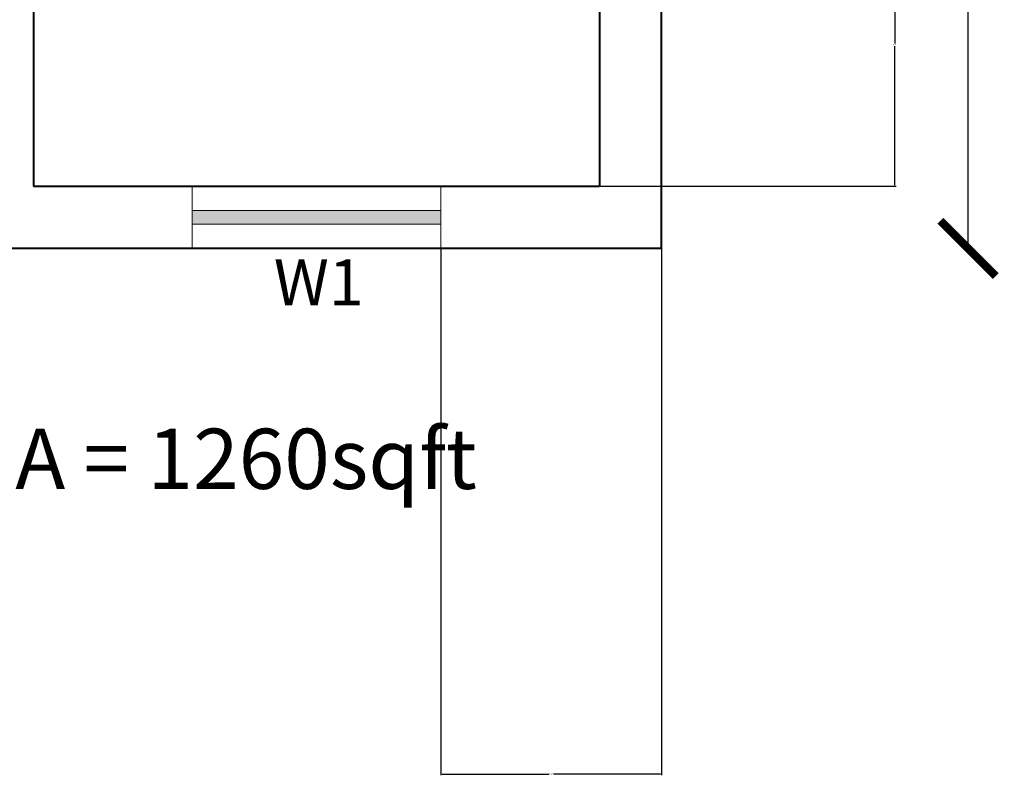
# Model space of a CAD drawing. Units: inches. Extents: x 182 to 1022, y -617 to 111.
# Tile 24 of 33: x 879 to 1022, y -617 to -507. Entities that reach past the tile are written whole.
import ezdxf

# ---------------------------------------------------------------- set-up
doc = ezdxf.new("R2010")
doc.units = ezdxf.units.IN
doc.header["$MEASUREMENT"] = 0
for name, color, linetype, lineweight in [('A-ANNO-DIMS', 2, 'Continuous', 18), ('A-ANNO-IDEN', 1, 'Continuous', 18), ('A-ANNO-TEXT', 8, 'Continuous', 20), ('A-GLAZ-PATT', 5, 'Continuous', 13), ('wall', 1, 'Continuous', 40), ('wind', 5, 'Continuous', 20)]:
    doc.layers.add(name, color=color, linetype=linetype, lineweight=lineweight)
doc.styles.get("Standard").update_dxf_attribs({"font": 'arial.ttf'})
doc.dimstyles.get("Standard").update_dxf_attribs({"dimtxt": 0.18, "dimasz": 0.18, "dimexe": 0.18, "dimexo": 0.0625, "dimgap": 0.09, "dimtad": 0, "dimtih": 1, "dimtoh": 1, "dimdec": 1, "dimzin": 0, "dimdsep": 46, "dimlunit": 4, "dimtxsty": 'Standard', "dimcen": 0.09, "dimadec": 0, "dimazin": 0, "dimtfac": 1, "dimtdec": 1, "dimtofl": 0, "dimtmove": 0, "dimatfit": 3, "dimfxl": 1, "dimtolj": 1, "dimtzin": 0, "dimarcsym": 0})

# ---------------------------------------------------------------- blocks, each defined once
blk = doc.blocks.new('_ArchTick')
at = {"color": 0, "linetype": 'ByBlock', "const_width": 0.15}
blk.add_lwpolyline([(-0.5, -0.5), (0.5, 0.5)], dxfattribs=at)
blk = doc.blocks.new('*D8')
at = {"layer": 'A-ANNO-DIMS', "color": 0, "lineweight": -2, "transparency": 16777216}
for p, q in [((1016.69, -0.37), (1016.69, -260.42)), ((1016.69, -540.37), (1016.69, -280.32))]:
    blk.add_line(p, q, dxfattribs=at)
at = {"layer": 'Defpoints', "color": 0, "transparency": 16777216}
for p in [(972.3, -0.37), (972.3, -540.37), (1016.69, -540.37)]:
    blk.add_point(p, dxfattribs=at)
at = {"layer": 'A-ANNO-DIMS', "color": 0, "lineweight": -2, "transparency": 16777216, "xscale": 8, "yscale": 8, "zscale": 8}
for p, rotation in [((1016.69, -0.37), 90), ((1016.69, -540.37), 270)]:
    blk.add_blockref('_ArchTick', p, dxfattribs=dict(at, rotation=rotation))
at = {"layer": 'A-ANNO-DIMS', "color": 0, "transparency": 16777216, "insert": (1016.69, -270.37), "char_height": 8, "attachment_point": 5, "rotation": 90}
blk.add_mtext("\\A1;45'", dxfattribs=at)
blk = doc.blocks.new('*D40')
at = {"layer": 'A-ANNO-DIMS', "color": 0, "lineweight": -2, "transparency": 16777216}
for p, q in [((940.3, -540.44), (940.3, -616.67)), ((972.3, -540.44), (972.3, -616.67)), ((940.48, -616.49), (955.97, -616.49)), ((972.12, -616.49), (956.64, -616.49))]:
    blk.add_line(p, q, dxfattribs=at)
at = {"layer": 'A-ANNO-DIMS', "color": 0, "transparency": 16777216}
for points in [[(940.48, -616.46), (940.48, -616.52), (940.3, -616.49)], [(972.12, -616.46), (972.12, -616.52), (972.3, -616.49)]]:
    blk.add_solid(points, dxfattribs=at)
at = {"layer": 'Defpoints', "color": 0, "transparency": 16777216}
for p in [(940.3, -540.37), (972.3, -540.37), (972.3, -616.49)]:
    blk.add_point(p, dxfattribs=at)
at = {"layer": 'A-ANNO-DIMS', "color": 0, "transparency": 16777216, "insert": (956.3, -616.49), "char_height": 0.18, "attachment_point": 5}
blk.add_mtext('\\A1;2\'-8"', dxfattribs=at)
blk = doc.blocks.new('*D45')
at = {"layer": 'A-ANNO-DIMS', "color": 0, "lineweight": -2, "transparency": 16777216}
for p, q in [((963.37, -490.37), (1006.28, -490.37)), ((1006.1, -490.55), (1006.1, -510.69)), ((1006.1, -531.19), (1006.1, -511.06)), ((963.37, -531.37), (1006.28, -531.37))]:
    blk.add_line(p, q, dxfattribs=at)
at = {"layer": 'A-ANNO-DIMS', "color": 0, "transparency": 16777216}
for points in [[(1006.07, -490.55), (1006.13, -490.55), (1006.1, -490.37)], [(1006.07, -531.19), (1006.13, -531.19), (1006.1, -531.37)]]:
    blk.add_solid(points, dxfattribs=at)
at = {"layer": 'Defpoints', "color": 0, "transparency": 16777216}
for p in [(963.3, -490.37), (963.3, -531.37), (1006.1, -531.37)]:
    blk.add_point(p, dxfattribs=at)
at = {"layer": 'A-ANNO-DIMS', "color": 0, "transparency": 16777216, "insert": (1006.1, -510.87), "char_height": 0.18, "attachment_point": 5}
blk.add_mtext('\\A1;3\'-5"', dxfattribs=at)

msp = doc.modelspace()

# ---------------------------------------------------------------- hatches: boundary and pattern name
at = {"layer": 'A-GLAZ-PATT'}
h = msp.add_hatch(color=256, dxfattribs=at)
h.dxf.hatch_style = 1
h.paths.add_polyline_path([(692.35, -3.87), (662.35, -3.87), (662.35, -5.87), (692.35, -5.87)])
h.paths.add_polyline_path([(783.03, -3.87), (747.03, -3.87), (747.03, -5.87), (783.03, -5.87)])
h.paths.add_polyline_path([(641.8, -252.37), (639.8, -252.37), (639.8, -288.37), (641.8, -288.37)])
h.paths.add_polyline_path([(968.8, -258.37), (966.8, -258.37), (966.8, -282.37), (968.8, -282.37)])
h.paths.add_polyline_path([(968.8, -132.92), (966.8, -132.92), (966.8, -168.92), (968.8, -168.92)])
h.paths.add_polyline_path([(940.3, -534.87), (904.3, -534.87), (904.3, -536.87), (940.3, -536.87)])

# ---------------------------------------------------------------- linework, layer by layer
at = {"layer": 'wall'}
for p, q in [((972.3, -540.37), (972.3, -0.37)), ((963.3, -322.87), (963.3, -531.37)), ((881.3, -396.37), (881.3, -531.37)), ((881.3, -531.37), (963.3, -531.37)), ((972.3, -540.37), (636.3, -540.37))]:
    msp.add_line(p, q, dxfattribs=at)
at = {"layer": 'wind'}
for p, q in [((904.3, -531.37), (904.3, -540.37)), ((940.3, -531.37), (940.3, -540.37)), ((904.3, -534.87), (940.3, -534.87)), ((904.3, -536.87), (940.3, -536.87))]:
    msp.add_line(p, q, dxfattribs=at)

# ---------------------------------------------------------------- texts
at = {"layer": 'A-ANNO-IDEN'}
msp.add_text('W1', height=6.652, dxfattribs=at).set_placement((916.12, -548.62))
at = {"layer": 'A-ANNO-TEXT', "insert": (764.16, -566.48), "char_height": 8.7185, "attachment_point": 1}
msp.add_mtext_dynamic_manual_height_columns('TOTAL BUILDUP AREA = 1260sqft', width=195.6714, gutter_width=1.45, heights=[0], dxfattribs=at)

# ---------------------------------------------------------------- dimensions: what is measured, and where the dimension line sits
at = {"layer": 'A-ANNO-DIMS'}
for base, p1, p2, angle, override, picture, middle in [((1016.69, -540.37), (972.3, -0.37), (972.3, -540.37), 90, {"dimtxt": 8, "dimasz": 8, "dimgap": 3, "dimtih": 0, "dimblk1": 'ArchTick', "dimblk2": 'ArchTick', "dimsah": 1, "dimse1": 1, "dimse2": 1, "dimclrd": 0, "dimclre": 0, "dimclrt": 0}, '*D8', (1016.69, -270.37)), ((1006.1, -531.37), (963.3, -490.37), (963.3, -531.37), 270, {"dimdec": 1, "dimlfac": 1, "dimrnd": 0, "dimzin": 1, "dimdsep": 46, "dimlunit": 4, "dimfrac": 2}, '*D45', (1006.1, -510.87))]:
    dim = msp.add_linear_dim(base=base, p1=p1, p2=p2, angle=angle, dimstyle='Standard', override=override, dxfattribs=at)
    dim.commit()
    dim.dimension.update_dxf_attribs({"geometry": picture, "text_midpoint": middle})
dim = msp.add_linear_dim(base=(972.3, -616.49), p1=(940.3, -540.37), p2=(972.3, -540.37), dimstyle='Standard', override={"dimdec": 1, "dimlfac": 1, "dimrnd": 0, "dimzin": 1, "dimdsep": 46, "dimlunit": 4, "dimfrac": 2}, dxfattribs=at)
dim.commit()
dim.dimension.update_dxf_attribs({"geometry": '*D40', "text_midpoint": (956.3, -616.49)})

doc.saveas('drawing.dxf')
